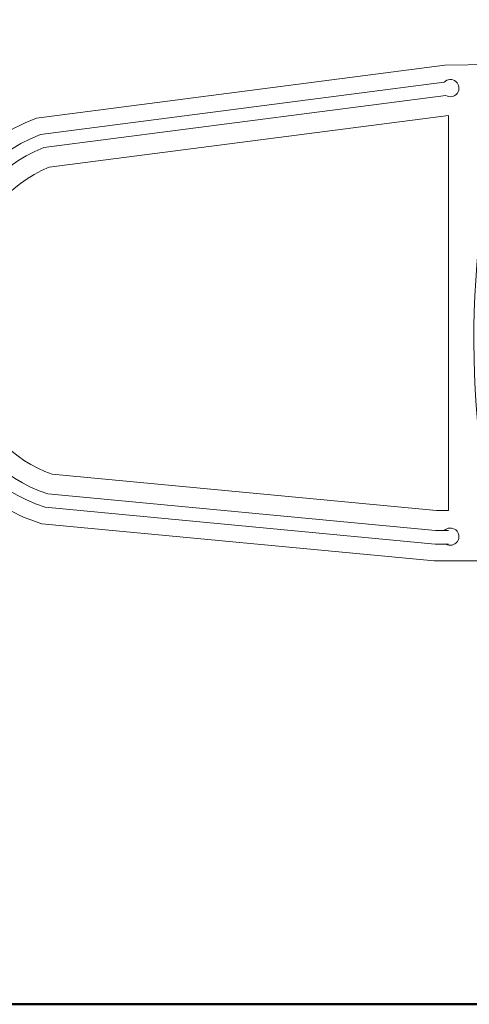
# Model space of a CAD drawing. Units: inches. Extents: x 64 to 1167, y 117 to 939.
# Tile 7 of 56: x 210 to 226, y 585 to 619. Entities that reach past the tile are written whole.
import ezdxf

# ---------------------------------------------------------------- set-up
doc = ezdxf.new("R2010")
doc.units = ezdxf.units.IN
doc.header["$MEASUREMENT"] = 0
doc.layers.add('A-FLOR-FIXT', color=8, linetype='Continuous', lineweight=18)
doc.layers.add('A-WALL', color=7, linetype='Continuous', lineweight=50)

# ---------------------------------------------------------------- blocks, each defined once
blk = doc.blocks.new('A$C2B992F40')
for p, q in [((39.23, 615.24), (39.23, 696.15)), ((39.23, 696.15), (475.68, 696.15)), ((66.85, 669.73), (39.23, 696.15)), ((444.23, 669.73), (475.68, 696.15)), ((475.68, 696.15), (475.68, 509.8)), ((66.85, 534.62), (66.85, 669.73)), ((66.85, 669.73), (444.23, 669.73)), ((444.23, 669.73), (444.23, 534.62)), ((0, 561.3), (0, 615.24)), ((0, 615.24), (51.49, 615.24)), ((51.49, 615.24), (51.49, 556.39)), ((51.49, 556.39), (39.23, 553.94)), ((39.23, 522.06), (39.23, 553.94)), ((444.23, 534.62), (66.85, 534.62)), ((40.06, 461.24), (39.23, 522.06)), ((475.68, 509.8), (475.68, 451.92)), ((86.65, 102.5), (40.06, 461.24)), ((101.02, 106.05), (54.98, 460.61)), ((112.51, 108.95), (66.65, 462.12)), ((84.15, 464.39), (431.55, 464.39)), ((129.73, 113.43), (84.15, 464.39)), ((431.55, 464.39), (431.55, 454.01)), ((449.2, 464.39), (449.2, 453.17)), ((460.97, 464.39), (460.97, 452.62)), ((431.55, 454.01), (399.59, 116.19)), ((449.2, 453.17), (416.97, 112.48)), ((460.97, 452.62), (428.57, 110.08)), ((475.68, 451.92), (443.06, 107.16)), ((324.19, 44.13), (215, 44.13)), ((326.66, 26.48), (213.44, 26.48)), ((328.22, 14.71), (212.45, 14.71)), ((330.08, 0), (211.28, 0))]:
    blk.add_line(p, q)
for centre, radius, start, end in [((22.2, 571.41), 24.4, 204.49972, 314.26101), ((280.26, 1327.83), 841.04, 253.34642, 283.43557), ((60.2, 466.07), 7.56, 328.52932, 226.26991), ((454.43, 466.07), 7.56, 328.52932, 226.26991), ((235.93, 157), 114.79, 202.30203, 259.4948), ((291.54, 153.78), 114.41, 286.5809, 340.81554), ((235.93, 157), 144.21, 200.68762, 260.63012), ((235.93, 157), 132.44, 201.26818, 260.22173), ((291.54, 153.78), 132.06, 285.42576, 341.7737), ((291.54, 153.78), 143.83, 284.77755, 342.31156), ((291.54, 153.78), 158.54, 284.07165, 342.89742), ((235.93, 157), 158.92, 200.05507, 261.07522)]:
    blk.add_arc(centre, radius, start, end)

msp = doc.modelspace()

# ---------------------------------------------------------------- linework, layer by layer
at = {"layer": 'A-WALL'}
msp.add_line((255.107, 585.2), (165.276, 585.2), dxfattribs=at)

# ---------------------------------------------------------------- block references
at = {"layer": 'A-FLOR-FIXT', "xscale": 0.0393700787401575, "yscale": 0.0393700787401575, "zscale": 0.0393700787401575, "rotation": 270.0000000000154}
msp.add_blockref('A$C2B992F40', (206.919, 619.278), dxfattribs=at)

doc.saveas('drawing.dxf')
